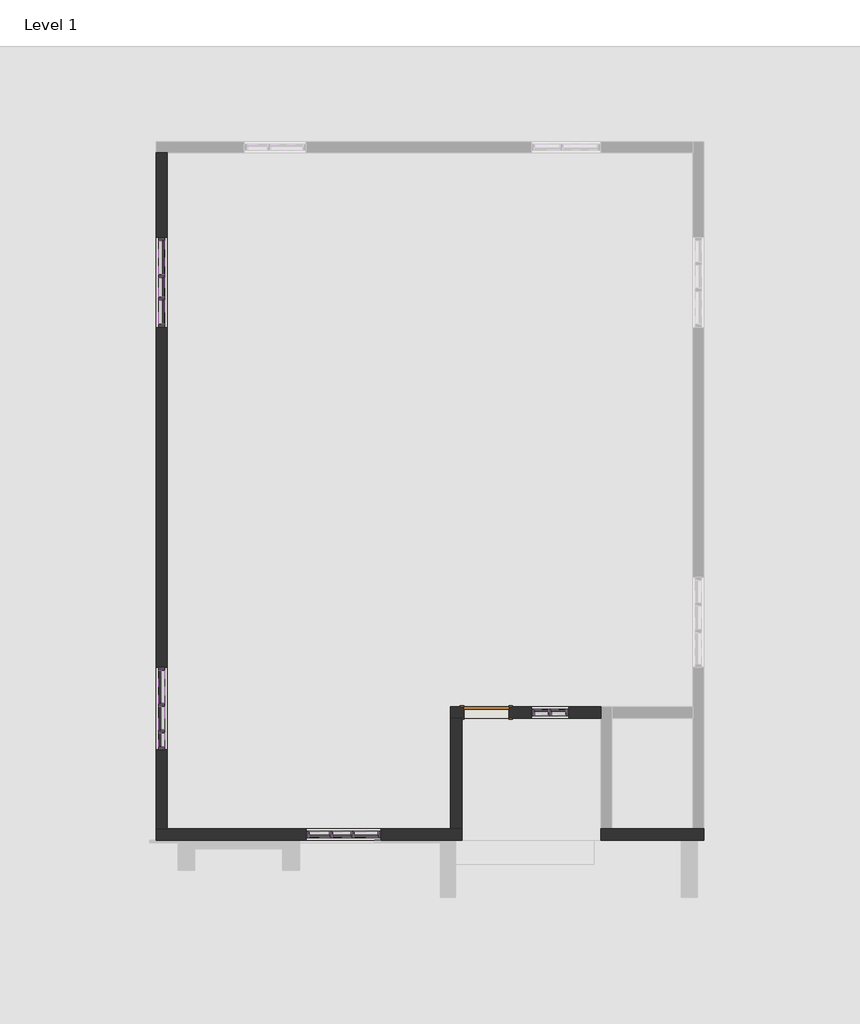
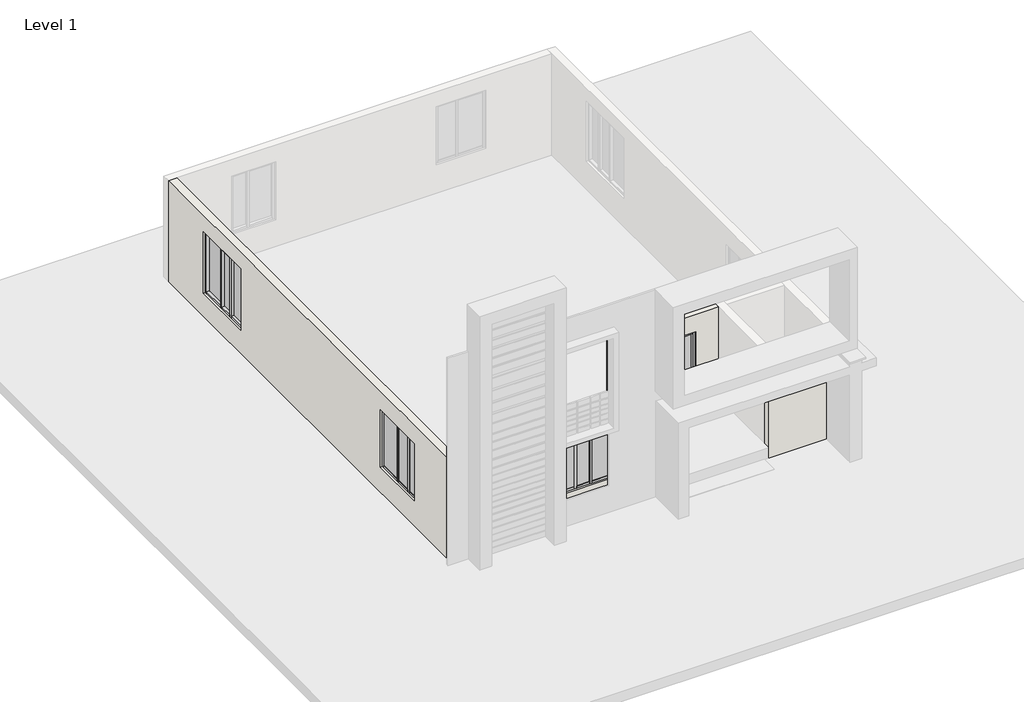
# One storey, part 1 of 2: 37 members, 11 plates, 5 walls, 1 door.
"""IFC4 building model written with IfcOpenShell, lengths in millimetres."""

from ifc_helpers import new_model, si_unit, frame, origin, origin_with_axes, place, context, project, spatial, polyline, outline, extrude, faceted_brep, transform, mapped, element, save
from components import door_a90ba1ad, member_b9f3750b, member_83c59054, member_dc106669, member_de80672f, member_ef20d1bc, member_6c34f49c, member_dac5616b, member_876c57a8, member_2b79973d, member_c33c434a, member_7096a90e, member_5f1d7e17, member_bcae55ac, member_51608f29, member_481990fb, member_106fc096, system_panel_glazed_5c179d98, system_panel_glazed_76585487, system_panel_glazed_8729007e, system_panel_glazed_f1a934e3, system_panel_glazed_8f71a385, system_panel_glazed_27f64093, system_panel_glazed_a2b4c657, system_panel_glazed_6f8e0303, system_panel_glazed_ba9a01dc, system_panel_glazed_7060130a

model = new_model("IFC4")

# Units and contexts
model_context = context("Model", 3, world=origin())
ifc_project = project(units=[si_unit("LENGTHUNIT", "METRE", prefix="MILLI")], contexts=[model_context])

# Site, building, storey
site = spatial("IfcSite", under=ifc_project)
building = spatial("IfcBuilding", under=site)
storey = spatial("IfcBuildingStorey", under=building, Name="Level 1", Elevation=0.0)

# Door
placement = place(None, origin())
door_shape = door_a90ba1ad(model_context)
element("IfcDoor", 1, ObjectType="Single-Flush : 36\" x 84\"", at=placement, inside=storey, context=model_context, shape_type="MappedRepresentation", body=[
    mapped(door_shape, transform((-10024.7281629, -12258.1678064, 355.6), x_axis=(-1.0, 0.0, 0.0), y_axis=(0.0, -1.0, 0.0), z_axis=(0.0, 0.0, 1.0))),
])

# Members
member_shape = member_b9f3750b(model_context)
element("IfcMember", 2, ObjectType="Rectangular Mullion : 2.5\" x 5\" rectangular", at=placement, inside=storey, context=model_context, shape_type="MappedRepresentation", body=[
    mapped(member_shape, transform((-12710.7781629, -14734.6678064, 2721.859847), x_axis=(0.0, 0.0, 1.0), y_axis=(0.0, 1.0, 0.0), z_axis=(-1.0, 0.0, 0.0))),
])
element("IfcMember", 3, ObjectType="Rectangular Mullion : 2.5\" x 5\" rectangular", at=placement, inside=storey, context=model_context, shape_type="MappedRepresentation", body=[
    mapped(member_shape, transform((-16616.0281629, -4384.1678064, 2553.8561304), x_axis=(0.0, 0.0, 1.0), y_axis=(-1.0, 0.0, 0.0), z_axis=(0.0, -1.0, 0.0))),
])
member_2_shape = member_83c59054(model_context)
element("IfcMember", 4, ObjectType="Rectangular Mullion : 2.5\" x 5\" rectangular", at=placement, inside=storey, context=model_context, shape_type="MappedRepresentation", body=[
    mapped(member_2_shape, transform((-13142.5781629, -14734.6678064, 2721.859847), x_axis=(0.0, 0.0, 1.0), y_axis=(0.0, 1.0, 0.0), z_axis=(-1.0, 0.0, 0.0))),
])
member_3_shape = member_dc106669(model_context)
element("IfcMember", 5, ObjectType="Rectangular Mullion : 2.5\" x 5\" rectangular", at=placement, inside=storey, context=model_context, shape_type="MappedRepresentation", body=[
    mapped(member_3_shape, transform((-13618.8281629, -14734.6678064, 2721.859847), x_axis=(0.0, 0.0, 1.0), y_axis=(0.0, 1.0, 0.0), z_axis=(-1.0, 0.0, 0.0))),
])
member_4_shape = member_de80672f(model_context)
element("IfcMember", 6, ObjectType="Rectangular Mullion : 2.5\" x 5\" rectangular", at=placement, inside=storey, context=model_context, shape_type="MappedRepresentation", body=[
    mapped(member_4_shape, transform((-13174.3281629, -14734.6678064, 964.766173), x_axis=(-1.0, 0.0, 0.0), y_axis=(0.0, 1.0, 0.0), z_axis=(0.0, 0.0, -1.0))),
])
element("IfcMember", 7, ObjectType="Rectangular Mullion : 2.5\" x 5\" rectangular", at=placement, inside=storey, context=model_context, shape_type="MappedRepresentation", body=[
    mapped(member_4_shape, transform((-12742.5281629, -14734.6678064, 964.766173), x_axis=(-1.0, 0.0, 0.0), y_axis=(0.0, 1.0, 0.0), z_axis=(0.0, 0.0, -1.0))),
])
element("IfcMember", 8, ObjectType="Rectangular Mullion : 2.5\" x 5\" rectangular", at=placement, inside=storey, context=model_context, shape_type="MappedRepresentation", body=[
    mapped(member_2_shape, transform((-12774.2781629, -14734.6678064, 964.766173), x_axis=(0.0, 0.0, -1.0), y_axis=(0.0, 1.0, 0.0), z_axis=(1.0, 0.0, 0.0))),
])
element("IfcMember", 9, ObjectType="Rectangular Mullion : 2.5\" x 5\" rectangular", at=placement, inside=storey, context=model_context, shape_type="MappedRepresentation", body=[
    mapped(member_3_shape, transform((-13206.0781629, -14734.6678064, 964.766173), x_axis=(0.0, 0.0, -1.0), y_axis=(0.0, 1.0, 0.0), z_axis=(1.0, 0.0, 0.0))),
])
element("IfcMember", 10, ObjectType="Rectangular Mullion : 2.5\" x 5\" rectangular", at=placement, inside=storey, context=model_context, shape_type="MappedRepresentation", body=[
    mapped(member_shape, transform((-12221.8281629, -14734.6678064, 964.766173), x_axis=(0.0, 0.0, -1.0), y_axis=(0.0, 1.0, 0.0), z_axis=(1.0, 0.0, 0.0))),
])
element("IfcMember", 11, ObjectType="Rectangular Mullion : 2.5\" x 5\" rectangular", at=placement, inside=storey, context=model_context, shape_type="MappedRepresentation", body=[
    mapped(member_shape, transform((-16616.0281629, -3895.2178064, 701.0746758), x_axis=(0.0, 0.0, -1.0), y_axis=(-1.0, 0.0, 0.0), z_axis=(0.0, 1.0, 0.0))),
])
member_5_shape = member_ef20d1bc(model_context)
element("IfcMember", 12, ObjectType="Rectangular Mullion : 2.5\" x 5\" rectangular", at=placement, inside=storey, context=model_context, shape_type="MappedRepresentation", body=[
    mapped(member_5_shape, transform((-13682.3281629, -14734.6678064, 964.766173), x_axis=(-1.0, 0.0, 0.0), y_axis=(0.0, 1.0, 0.0), z_axis=(0.0, 0.0, -1.0))),
])
element("IfcMember", 13, ObjectType="Rectangular Mullion : 2.5\" x 5\" rectangular", at=placement, inside=storey, context=model_context, shape_type="MappedRepresentation", body=[
    mapped(member_5_shape, transform((-12158.3281629, -14734.6678064, 2721.859847), x_axis=(1.0, 0.0, 0.0), y_axis=(0.0, 1.0, 0.0), z_axis=(0.0, 0.0, 1.0))),
])
member_6_shape = member_6c34f49c(model_context)
element("IfcMember", 14, ObjectType="Rectangular Mullion : 2.5\" x 5\" rectangular", at=placement, inside=storey, context=model_context, shape_type="MappedRepresentation", body=[
    mapped(member_6_shape, transform((-8761.0781629, -12258.1678064, 2518.9925001), x_axis=(0.0, 0.0, 1.0), y_axis=(0.0, -1.0, 0.0), z_axis=(1.0, 0.0, 0.0))),
])
element("IfcMember", 15, ObjectType="Rectangular Mullion : 2.5\" x 5\" rectangular", at=placement, inside=storey, context=model_context, shape_type="MappedRepresentation", body=[
    mapped(member_6_shape, transform((-8411.8281629, -12258.1678064, 2518.9925001), x_axis=(0.0, 0.0, 1.0), y_axis=(0.0, -1.0, 0.0), z_axis=(1.0, 0.0, 0.0))),
])
element("IfcMember", 16, ObjectType="Rectangular Mullion : 2.5\" x 5\" rectangular", at=placement, inside=storey, context=model_context, shape_type="MappedRepresentation", body=[
    mapped(member_6_shape, transform((-16616.0281629, -12670.9178064, 2484.9814281), x_axis=(0.0, 0.0, 1.0), y_axis=(1.0, 0.0, 0.0), z_axis=(0.0, 1.0, 0.0))),
])
member_7_shape = member_dac5616b(model_context)
element("IfcMember", 17, ObjectType="Rectangular Mullion : 2.5\" x 5\" rectangular", at=placement, inside=storey, context=model_context, shape_type="MappedRepresentation", body=[
    mapped(member_7_shape, transform((-8729.3281629, -12258.1678064, 782.9762742), x_axis=(1.0, 0.0, 0.0), y_axis=(0.0, -1.0, 0.0), z_axis=(0.0, 0.0, -1.0))),
])
element("IfcMember", 18, ObjectType="Rectangular Mullion : 2.5\" x 5\" rectangular", at=placement, inside=storey, context=model_context, shape_type="MappedRepresentation", body=[
    mapped(member_6_shape, transform((-8697.5781629, -12258.1678064, 782.9762742), x_axis=(0.0, 0.0, -1.0), y_axis=(0.0, -1.0, 0.0), z_axis=(-1.0, 0.0, 0.0))),
])
element("IfcMember", 19, ObjectType="Rectangular Mullion : 2.5\" x 5\" rectangular", at=placement, inside=storey, context=model_context, shape_type="MappedRepresentation", body=[
    mapped(member_6_shape, transform((-9046.8281629, -12258.1678064, 782.9762742), x_axis=(0.0, 0.0, -1.0), y_axis=(0.0, -1.0, 0.0), z_axis=(-1.0, 0.0, 0.0))),
])
element("IfcMember", 20, ObjectType="Rectangular Mullion : 2.5\" x 5\" rectangular", at=placement, inside=storey, context=model_context, shape_type="MappedRepresentation", body=[
    mapped(member_6_shape, transform((-16616.0281629, -12956.6678064, 764.9931836), x_axis=(0.0, 0.0, -1.0), y_axis=(1.0, 0.0, 0.0), z_axis=(0.0, -1.0, 0.0))),
])
member_8_shape = member_876c57a8(model_context)
element("IfcMember", 21, ObjectType="Rectangular Mullion : 2.5\" x 5\" rectangular", at=placement, inside=storey, context=model_context, shape_type="MappedRepresentation", body=[
    mapped(member_8_shape, transform((-8348.3281629, -12258.1678064, 782.9762742), x_axis=(1.0, 0.0, 0.0), y_axis=(0.0, -1.0, 0.0), z_axis=(0.0, 0.0, -1.0))),
])
element("IfcMember", 22, ObjectType="Rectangular Mullion : 2.5\" x 5\" rectangular", at=placement, inside=storey, context=model_context, shape_type="MappedRepresentation", body=[
    mapped(member_8_shape, transform((-9110.3281629, -12258.1678064, 2518.9925001), x_axis=(-1.0, 0.0, 0.0), y_axis=(0.0, -1.0, 0.0), z_axis=(0.0, 0.0, 1.0))),
])
member_9_shape = member_2b79973d(model_context)
element("IfcMember", 23, ObjectType="Rectangular Mullion : 2.5\" x 5\" rectangular", at=placement, inside=storey, context=model_context, shape_type="MappedRepresentation", body=[
    mapped(member_9_shape, transform((-16616.0281629, -12137.5178064, 2484.9814281), x_axis=(0.0, 0.0, 1.0), y_axis=(1.0, 0.0, 0.0), z_axis=(0.0, 1.0, 0.0))),
])
member_10_shape = member_c33c434a(model_context)
element("IfcMember", 24, ObjectType="Rectangular Mullion : 2.5\" x 5\" rectangular", at=placement, inside=storey, context=model_context, shape_type="MappedRepresentation", body=[
    mapped(member_10_shape, transform((-16616.0281629, -11407.2678064, 2484.9814281), x_axis=(0.0, 0.0, 1.0), y_axis=(1.0, 0.0, 0.0), z_axis=(0.0, 1.0, 0.0))),
])
element("IfcMember", 25, ObjectType="Rectangular Mullion : 2.5\" x 5\" rectangular", at=placement, inside=storey, context=model_context, shape_type="MappedRepresentation", body=[
    mapped(member_9_shape, transform((-16616.0281629, -12607.4178064, 764.9931836), x_axis=(0.0, 0.0, -1.0), y_axis=(1.0, 0.0, 0.0), z_axis=(0.0, -1.0, 0.0))),
])
element("IfcMember", 26, ObjectType="Rectangular Mullion : 2.5\" x 5\" rectangular", at=placement, inside=storey, context=model_context, shape_type="MappedRepresentation", body=[
    mapped(member_10_shape, transform((-16616.0281629, -12074.0178064, 764.9931836), x_axis=(0.0, 0.0, -1.0), y_axis=(1.0, 0.0, 0.0), z_axis=(0.0, -1.0, 0.0))),
])
member_11_shape = member_7096a90e(model_context)
element("IfcMember", 27, ObjectType="Rectangular Mullion : 2.5\" x 5\" rectangular", at=placement, inside=storey, context=model_context, shape_type="MappedRepresentation", body=[
    mapped(member_11_shape, transform((-16616.0281629, -3831.7178064, 2553.8561304), x_axis=(0.0, 0.0, 1.0), y_axis=(-1.0, 0.0, 0.0), z_axis=(0.0, -1.0, 0.0))),
])
member_12_shape = member_5f1d7e17(model_context)
element("IfcMember", 28, ObjectType="Rectangular Mullion : 2.5\" x 5\" rectangular", at=placement, inside=storey, context=model_context, shape_type="MappedRepresentation", body=[
    mapped(member_12_shape, transform((-16616.0281629, -3374.5178064, 2553.8561304), x_axis=(0.0, 0.0, 1.0), y_axis=(-1.0, 0.0, 0.0), z_axis=(0.0, -1.0, 0.0))),
])
member_13_shape = member_bcae55ac(model_context)
element("IfcMember", 29, ObjectType="Rectangular Mullion : 2.5\" x 5\" rectangular", at=placement, inside=storey, context=model_context, shape_type="MappedRepresentation", body=[
    mapped(member_13_shape, transform((-16616.0281629, -3406.2678064, 701.0746758), x_axis=(0.0, -1.0, 0.0), y_axis=(-1.0, 0.0, 0.0), z_axis=(0.0, 0.0, -1.0))),
])
element("IfcMember", 30, ObjectType="Rectangular Mullion : 2.5\" x 5\" rectangular", at=placement, inside=storey, context=model_context, shape_type="MappedRepresentation", body=[
    mapped(member_13_shape, transform((-16616.0281629, -3863.4678064, 701.0746758), x_axis=(0.0, -1.0, 0.0), y_axis=(-1.0, 0.0, 0.0), z_axis=(0.0, 0.0, -1.0))),
])
element("IfcMember", 31, ObjectType="Rectangular Mullion : 2.5\" x 5\" rectangular", at=placement, inside=storey, context=model_context, shape_type="MappedRepresentation", body=[
    mapped(member_11_shape, transform((-16616.0281629, -3438.0178064, 701.0746758), x_axis=(0.0, 0.0, -1.0), y_axis=(-1.0, 0.0, 0.0), z_axis=(0.0, 1.0, 0.0))),
])
element("IfcMember", 32, ObjectType="Rectangular Mullion : 2.5\" x 5\" rectangular", at=placement, inside=storey, context=model_context, shape_type="MappedRepresentation", body=[
    mapped(member_12_shape, transform((-16616.0281629, -2682.3678064, 701.0746758), x_axis=(0.0, 0.0, -1.0), y_axis=(-1.0, 0.0, 0.0), z_axis=(0.0, 1.0, 0.0))),
])
member_14_shape = member_51608f29(model_context)
element("IfcMember", 33, ObjectType="Rectangular Mullion : 2.5\" x 5\" rectangular", at=placement, inside=storey, context=model_context, shape_type="MappedRepresentation", body=[
    mapped(member_14_shape, transform((-16616.0281629, -4447.6678064, 701.0746758), x_axis=(0.0, -1.0, 0.0), y_axis=(-1.0, 0.0, 0.0), z_axis=(0.0, 0.0, -1.0))),
])
element("IfcMember", 34, ObjectType="Rectangular Mullion : 2.5\" x 5\" rectangular", at=placement, inside=storey, context=model_context, shape_type="MappedRepresentation", body=[
    mapped(member_14_shape, transform((-16616.0281629, -2618.8678064, 2553.8561304), x_axis=(0.0, 1.0, 0.0), y_axis=(-1.0, 0.0, 0.0), z_axis=(0.0, 0.0, 1.0))),
])
member_15_shape = member_481990fb(model_context)
element("IfcMember", 35, ObjectType="Rectangular Mullion : 2.5\" x 5\" rectangular", at=placement, inside=storey, context=model_context, shape_type="MappedRepresentation", body=[
    mapped(member_15_shape, transform((-16616.0281629, -12105.7678064, 764.9931836), x_axis=(0.0, 1.0, 0.0), y_axis=(1.0, 0.0, 0.0), z_axis=(0.0, 0.0, -1.0))),
])
element("IfcMember", 36, ObjectType="Rectangular Mullion : 2.5\" x 5\" rectangular", at=placement, inside=storey, context=model_context, shape_type="MappedRepresentation", body=[
    mapped(member_15_shape, transform((-16616.0281629, -12639.1678064, 764.9931836), x_axis=(0.0, 1.0, 0.0), y_axis=(1.0, 0.0, 0.0), z_axis=(0.0, 0.0, -1.0))),
])
member_16_shape = member_106fc096(model_context)
element("IfcMember", 37, ObjectType="Rectangular Mullion : 2.5\" x 5\" rectangular", at=placement, inside=storey, context=model_context, shape_type="MappedRepresentation", body=[
    mapped(member_16_shape, transform((-16616.0281629, -13020.1678064, 2484.9814281), x_axis=(0.0, -1.0, 0.0), y_axis=(1.0, 0.0, 0.0), z_axis=(0.0, 0.0, 1.0))),
])
element("IfcMember", 38, ObjectType="Rectangular Mullion : 2.5\" x 5\" rectangular", at=placement, inside=storey, context=model_context, shape_type="MappedRepresentation", body=[
    mapped(member_16_shape, transform((-16616.0281629, -11343.7678064, 764.9931836), x_axis=(0.0, 1.0, 0.0), y_axis=(1.0, 0.0, 0.0), z_axis=(0.0, 0.0, -1.0))),
])

# Plates
system_panel_glazed_shape = system_panel_glazed_5c179d98(model_context)
element("IfcPlate", 39, ObjectType="System Panel : Glazed", at=placement, inside=storey, context=model_context, shape_type="MappedRepresentation", body=[
    mapped(system_panel_glazed_shape, transform((-12466.3031629, -14734.6678064, 1028.266173), x_axis=(-1.0, 0.0, 0.0), y_axis=(0.0, -1.0, 0.0), z_axis=(0.0, 0.0, 1.0))),
])
system_panel_glazed_2_shape = system_panel_glazed_76585487(model_context)
element("IfcPlate", 40, ObjectType="System Panel : Glazed", at=placement, inside=storey, context=model_context, shape_type="MappedRepresentation", body=[
    mapped(system_panel_glazed_2_shape, transform((-13412.4531629, -14734.6678064, 1028.266173), x_axis=(-1.0, 0.0, 0.0), y_axis=(0.0, -1.0, 0.0), z_axis=(0.0, 0.0, 1.0))),
])
system_panel_glazed_3_shape = system_panel_glazed_8729007e(model_context)
element("IfcPlate", 41, ObjectType="System Panel : Glazed", at=placement, inside=storey, context=model_context, shape_type="MappedRepresentation", body=[
    mapped(system_panel_glazed_3_shape, transform((-12958.4281629, -14734.6678064, 1028.266173), x_axis=(-1.0, 0.0, 0.0), y_axis=(0.0, -1.0, 0.0), z_axis=(0.0, 0.0, 1.0))),
])
system_panel_glazed_4_shape = system_panel_glazed_f1a934e3(model_context)
element("IfcPlate", 42, ObjectType="System Panel : Glazed", at=placement, inside=storey, context=model_context, shape_type="MappedRepresentation", body=[
    mapped(system_panel_glazed_4_shape, transform((-8903.9531629, -12258.1678064, 846.4762742), x_axis=(1.0, 0.0, 0.0), y_axis=(0.0, 1.0, 0.0), z_axis=(0.0, 0.0, 1.0))),
])
element("IfcPlate", 43, ObjectType="System Panel : Glazed", at=placement, inside=storey, context=model_context, shape_type="MappedRepresentation", body=[
    mapped(system_panel_glazed_4_shape, transform((-8554.7031629, -12258.1678064, 846.4762742), x_axis=(1.0, 0.0, 0.0), y_axis=(0.0, 1.0, 0.0), z_axis=(0.0, 0.0, 1.0))),
])
system_panel_glazed_5_shape = system_panel_glazed_8f71a385(model_context)
element("IfcPlate", 44, ObjectType="System Panel : Glazed", at=placement, inside=storey, context=model_context, shape_type="MappedRepresentation", body=[
    mapped(system_panel_glazed_5_shape, transform((-16616.0281629, -3028.4428064, 764.5746758), x_axis=(0.0, -1.0, 0.0), y_axis=(1.0, 0.0, 0.0), z_axis=(0.0, 0.0, 1.0))),
])
system_panel_glazed_6_shape = system_panel_glazed_27f64093(model_context)
element("IfcPlate", 45, ObjectType="System Panel : Glazed", at=placement, inside=storey, context=model_context, shape_type="MappedRepresentation", body=[
    mapped(system_panel_glazed_6_shape, transform((-16616.0281629, -3634.8678064, 764.5746758), x_axis=(0.0, -1.0, 0.0), y_axis=(1.0, 0.0, 0.0), z_axis=(0.0, 0.0, 1.0))),
])
system_panel_glazed_7_shape = system_panel_glazed_a2b4c657(model_context)
element("IfcPlate", 46, ObjectType="System Panel : Glazed", at=placement, inside=storey, context=model_context, shape_type="MappedRepresentation", body=[
    mapped(system_panel_glazed_7_shape, transform((-16616.0281629, -4139.6928064, 764.5746758), x_axis=(0.0, -1.0, 0.0), y_axis=(1.0, 0.0, 0.0), z_axis=(0.0, 0.0, 1.0))),
])
system_panel_glazed_8_shape = system_panel_glazed_6f8e0303(model_context)
element("IfcPlate", 47, ObjectType="System Panel : Glazed", at=placement, inside=storey, context=model_context, shape_type="MappedRepresentation", body=[
    mapped(system_panel_glazed_8_shape, transform((-16616.0281629, -12813.7928064, 828.4931836), x_axis=(0.0, 1.0, 0.0), y_axis=(-1.0, 0.0, 0.0), z_axis=(0.0, 0.0, 1.0))),
])
system_panel_glazed_9_shape = system_panel_glazed_ba9a01dc(model_context)
element("IfcPlate", 48, ObjectType="System Panel : Glazed", at=placement, inside=storey, context=model_context, shape_type="MappedRepresentation", body=[
    mapped(system_panel_glazed_9_shape, transform((-16616.0281629, -11740.6428064, 828.4931836), x_axis=(0.0, 1.0, 0.0), y_axis=(-1.0, 0.0, 0.0), z_axis=(0.0, 0.0, 1.0))),
])
system_panel_glazed_10_shape = system_panel_glazed_7060130a(model_context)
element("IfcPlate", 49, ObjectType="System Panel : Glazed", at=placement, inside=storey, context=model_context, shape_type="MappedRepresentation", body=[
    mapped(system_panel_glazed_10_shape, transform((-16616.0281629, -12372.4678064, 828.4931836), x_axis=(0.0, 1.0, 0.0), y_axis=(-1.0, 0.0, 0.0), z_axis=(0.0, 0.0, 1.0))),
])

# Walls
element("IfcWall", 50, ObjectType="9\"", at=placement, inside=storey, context=model_context, shape_type="Brep", body=[
    faceted_brep([(-16730.3281629, -14848.9678064, 0.0), (-10520.0281629, -14848.9678064, 0.0), (-10520.0281629, -14848.9678064, 3048.0), (-16730.3281629, -14848.9678064, 3048.0), (-12158.3281629, -14848.9678064, 2721.859847), (-12158.3281629, -14848.9678064, 964.766173), (-13682.3281629, -14848.9678064, 964.766173), (-13682.3281629, -14848.9678064, 2721.859847), (-10520.0281629, -14620.3678064, 0.0), (-10748.6281629, -14620.3678064, 0.0), (-16501.7281629, -14620.3678064, 0.0), (-16730.3281629, -14620.3678064, 0.0), (-16730.3281629, -14620.3678064, 3048.0), (-16501.7281629, -14620.3678064, 3048.0), (-10748.6281629, -14620.3678064, 3048.0), (-10520.0281629, -14620.3678064, 3048.0), (-12158.3281629, -14620.3678064, 964.766173), (-12158.3281629, -14620.3678064, 2721.859847), (-13682.3281629, -14620.3678064, 2721.859847), (-13682.3281629, -14620.3678064, 964.766173)], [[[0, 1, 2, 3], [4, 5, 6, 7]], [[8, 9, 10, 11, 12, 13, 14, 15], [16, 17, 18, 19]], [[1, 0, 11, 10, 9, 8]], [[2, 1, 8, 15]], [[3, 2, 15, 14, 13, 12]], [[0, 3, 12, 11]], [[16, 5, 4, 17]], [[17, 4, 7, 18]], [[18, 7, 6, 19]], [[5, 16, 19, 6]]]),
])
element("IfcWall", 51, ObjectType="9\"", at=placement, inside=storey, context=model_context, shape_type="SweptSolid", body=[
    extrude(outline(polyline([(-904.3678064, 0.0), (-14620.3678064, 0.0), (-14620.3678064, 3048.0), (-904.3678064, 3048.0), (-904.3678064, 0.0)]), holes=[polyline([(-2618.8678064, 701.0746758), (-2618.8678064, 2553.8561304), (-4447.6678064, 2553.8561304), (-4447.6678064, 701.0746758), (-2618.8678064, 701.0746758)]), polyline([(-13020.1678064, 2484.9814281), (-13020.1678064, 764.9931836), (-11343.7678064, 764.9931836), (-11343.7678064, 2484.9814281), (-13020.1678064, 2484.9814281)])]), frame((-16730.3281629, 0.0, 0.0), z_axis=(1.0, 0.0, 0.0), x_axis=(0.0, 1.0, 0.0)), (0.0, 0.0, 1.0), 228.6),
])
element("IfcWall", 52, ObjectType="9\"", at=placement, inside=storey, context=model_context, shape_type="Brep", body=[
    faceted_brep([(-7700.6281629, -12143.8678064, 0.0), (-10748.6281629, -12143.8678064, 0.0), (-10748.6281629, -12143.8678064, 3048.0), (-7700.6281629, -12143.8678064, 3048.0), (-9567.5281629, -12143.8678064, 355.6), (-9567.5281629, -12143.8678064, 2489.2), (-10481.9281629, -12143.8678064, 2489.2), (-10481.9281629, -12143.8678064, 355.6), (-9110.3281629, -12143.8678064, 2518.9925001), (-9110.3281629, -12143.8678064, 782.9762742), (-8348.3281629, -12143.8678064, 782.9762742), (-8348.3281629, -12143.8678064, 2518.9925001), (-10748.6281629, -12372.4678064, 0.0), (-10520.0281629, -12372.4678064, 0.0), (-7700.6281629, -12372.4678064, 0.0), (-7700.6281629, -12372.4678064, 3048.0), (-10520.0281629, -12372.4678064, 3048.0), (-10748.6281629, -12372.4678064, 3048.0), (-9567.5281629, -12372.4678064, 355.6), (-10481.9281629, -12372.4678064, 355.6), (-10481.9281629, -12372.4678064, 2489.2), (-9567.5281629, -12372.4678064, 2489.2), (-9110.3281629, -12372.4678064, 782.9762742), (-9110.3281629, -12372.4678064, 2518.9925001), (-8348.3281629, -12372.4678064, 2518.9925001), (-8348.3281629, -12372.4678064, 782.9762742)], [[[0, 1, 2, 3], [4, 5, 6, 7], [8, 9, 10, 11]], [[12, 13, 14, 15, 16, 17], [18, 19, 20, 21], [22, 23, 24, 25]], [[0, 3, 15, 14]], [[2, 1, 12, 17]], [[19, 18, 4, 7]], [[20, 19, 7, 6]], [[21, 20, 6, 5]], [[18, 21, 5, 4]], [[22, 9, 8, 23]], [[23, 8, 11, 24]], [[24, 11, 10, 25]], [[9, 22, 25, 10]], [[1, 0, 14, 13, 12]], [[3, 2, 17, 16, 15]]]),
])
element("IfcWall", 53, ObjectType="9\"", at=placement, inside=storey, context=model_context, shape_type="SweptSolid", body=[
    extrude(outline(polyline([(-10748.6281629, -14620.3678064), (-10748.6281629, -12372.4678064), (-10520.0281629, -12372.4678064), (-10520.0281629, -14620.3678064), (-10748.6281629, -14620.3678064)])), origin_with_axes(), (0.0, 0.0, 1.0), 3048.0),
])
element("IfcWall", 54, ObjectType="9\"", at=placement, inside=storey, context=model_context, shape_type="Brep", body=[
    faceted_brep([(-7700.6281629, -14848.9678064, 0.0), (-5605.1281629, -14848.9678064, 0.0), (-5605.1281629, -14848.9678064, 3048.0), (-7700.6281629, -14848.9678064, 3048.0), (-7700.6281629, -14620.3678064, 0.0), (-7700.6281629, -14620.3678064, 3048.0), (-7472.0281629, -14620.3678064, 3048.0), (-5833.7281629, -14620.3678064, 3048.0), (-5605.1281629, -14620.3678064, 3048.0), (-5605.1281629, -14620.3678064, 0.0), (-5833.7281629, -14620.3678064, 0.0), (-7472.0281629, -14620.3678064, 0.0)], [[[0, 1, 2, 3]], [[4, 5, 6, 7, 8, 9, 10, 11]], [[1, 0, 4, 11, 10, 9]], [[3, 2, 8, 7, 6, 5]], [[0, 3, 5, 4]], [[2, 1, 9, 8]]]),
])

save(model, "model.ifc")

# Revit data of these elements
# Type "Single-Flush : 36\" x 84\""
#   Type Mark = "1"
#   Construction Type Id = "MDOOR"
#   Assembly Code = "C1020"
#   Analytic Construction = "Metal"
#   Thickness = 0' - 2"
#   Heat Transfer Coefficient (U) = 0.651978 BTU/(h·ft²·°F)
#   Height = 7' - 0"
#   Trim Projection Ext = 0' - 1"
#   Trim Projection Int = 0' - 1"
#   Trim Width = 0' - 3"
#   Width = 3' - 0"
#   Define Thermal Properties by = 1
#   Define Thermal Properties by = 1
#   Door Material = Door - Panel
#   Frame Material = Door - Frame
#   Visual Light Transmittance = 0
#   Solar Heat Gain Coefficient = 0
#   Function = (empty or 0)
#   Wall Closure = (empty or 0)
# Type "Rectangular Mullion : 2.5\" x 5\" rectangular"
#   built-in parameter 1007304 = 0.416667 (stored number, unit not read)
#   built-in parameter 1007301 = 0.104167 (stored number, unit not read)
#   built-in parameter 1007300 = 0.104167 (stored number, unit not read)
# Type "System Panel : Glazed"
#   Construction Type Id = "GSP4R"
#   Analytic Construction = "1/8 in Pilkington single glazing"
#   Visual Light Transmittance = 0.9
#   Solar Heat Gain Coefficient = 0.86
#   Heat Transfer Coefficient (U) = 1.18115 BTU/(h·ft²·°F)
#   Define Thermal Properties by = 1
# Type "9\""
#   Assembly Code = "B2010"
#   Layers, outside or top first: 0' - 9" no material (function 1)
# Element 1 (IfcDoor, "Single-Flush : 36\" x 84\"")
#   Phase Created = New Construction
#   Materials on its faces: "Door - Frame", "Door - Panel"
# Elements 2, 3, 4, 5, 6, 7, 8, 9, 10, 11, 12, 13, 14, 15, 16, 17, 18, 19, 20, 21, 22, 23, 24, 25, 26, 27, 28, 29, 30, 31, 32, 33, 34, 35, 36, 37, 38 (IfcMember, "Rectangular Mullion : 2.5\" x 5\" rectangular")
#   Phase Created = New Construction
#   Materials on its faces: "Aluminum"
# Elements 39, 40, 41, 42, 43, 44, 45, 46, 47, 48, 49 (IfcPlate, "System Panel : Glazed")
#   Phase Created = New Construction
#   Materials on its faces: "Glass"
# Elements 50, 51, 52, 53, 54 (IfcWall, "9\"")
#   Top Offset = 0' - 0"
#   Base Offset = 0' - 0"
#   Unconnected Height = 10' - 0"
#   wall height = 10' - 0"
#   Phase Created = New Construction
#   Base Constraint = Level 1
#   Materials on its faces: "Default Wall"
# Materials
#   "Door - Panel": class "Wood", colour RGB 210 159 95, transparency 0, Cost = 0
#   "Door - Frame": colour RGB 118 70 51, transparency 0, Cost = 0
#   "Aluminum": class "Metal", colour RGB 247 247 247, transparency 0, Description = "Aluminum 6061", Cost = 0
#   "Glass": class "Glass", colour RGB 0 128 192, transparency 0.75, Description = "Soda Lime Glass", Cost = 0
#   "Default Wall": colour RGB 128 128 128, transparency 0, Cost = 0
